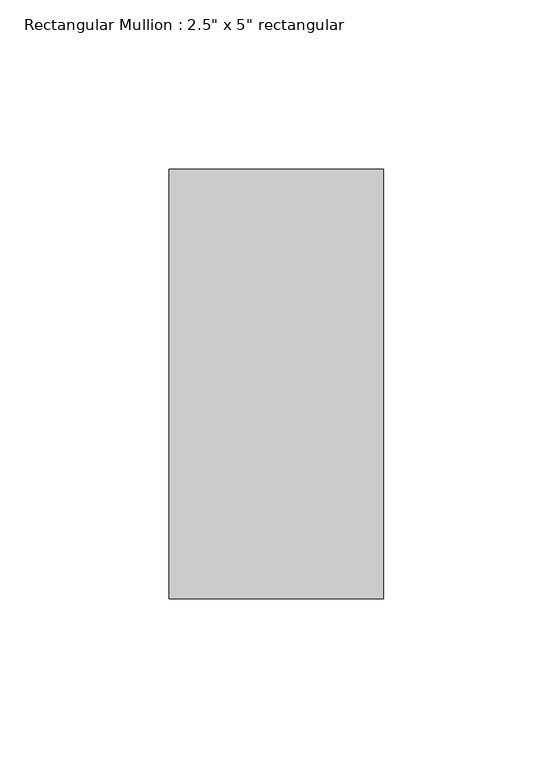
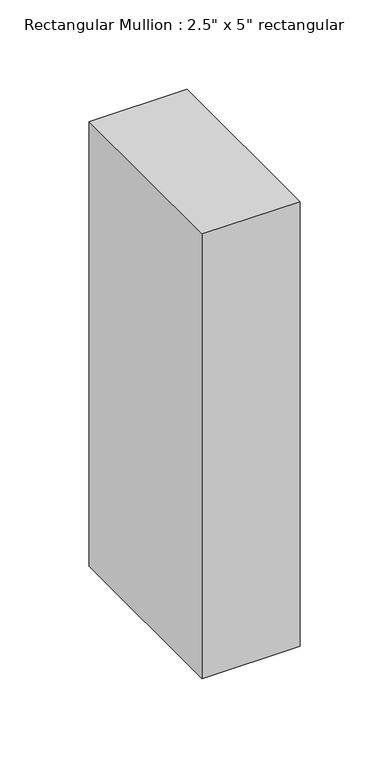
"""IFC4 building model written with IfcOpenShell, lengths in millimetres: member geometry."""

from ifc_helpers import new_model, si_unit, frame, origin, place, context, project, spatial, polyline, outline, extrude, source, transform, mapped, element, save


def member_75d1e245(model_context):
    return source(origin(), model_context, "Body", "SweptSolid", [
        extrude(outline(polyline([(31.75, 63.5), (31.75, -63.5), (-31.75, -63.5), (-31.75, 63.5), (31.75, 63.5)])), frame((0.0, 0.0, -304.8), z_axis=(0.0, 0.0, 1.0), x_axis=(1.0, 0.0, 0.0)), (0.0, 0.0, 1.0), 304.8),
    ])


if __name__ == "__main__":
    model = new_model("IFC4")
    model_context = context("Model", 3, world=origin())
    ifc_project = project(units=[si_unit("LENGTHUNIT", "METRE", prefix="MILLI")], contexts=[model_context])
    site = spatial("IfcSite", under=ifc_project)
    building = spatial("IfcBuilding", under=site)
    placement = place(None, origin())
    member_shape = member_75d1e245(model_context)
    element("IfcMember", 1, ObjectType="Rectangular Mullion : 2.5\" x 5\" rectangular", at=placement, inside=building, context=model_context, shape_type="MappedRepresentation", body=[
        mapped(member_shape, transform((0.0, 0.0, 0.0), x_axis=(1.0, 0.0, 0.0), y_axis=(0.0, 1.0, 0.0), z_axis=(0.0, 0.0, 1.0))),
    ])
    save(model, "model.ifc")

# Revit data of these elements
# Type "Rectangular Mullion : 2.5\" x 5\" rectangular"
#   built-in parameter 1007304 = 0.416667 (stored number, unit not read)
#   built-in parameter 1007301 = 0.104167 (stored number, unit not read)
#   built-in parameter 1007300 = 0.104167 (stored number, unit not read)
# Element 1 (IfcMember, "Rectangular Mullion : 2.5\" x 5\" rectangular")
#   Materials on its faces: "door colour"
# Materials
#   "door colour": class "Generic", colour RGB 120 120 120, transparency 0, Cost = 0
